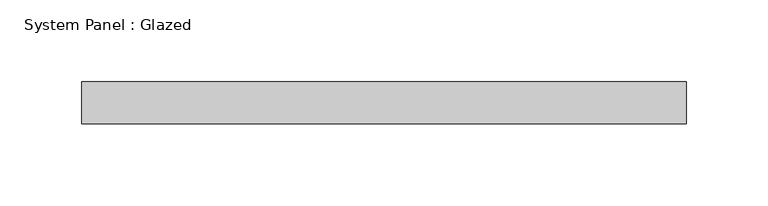
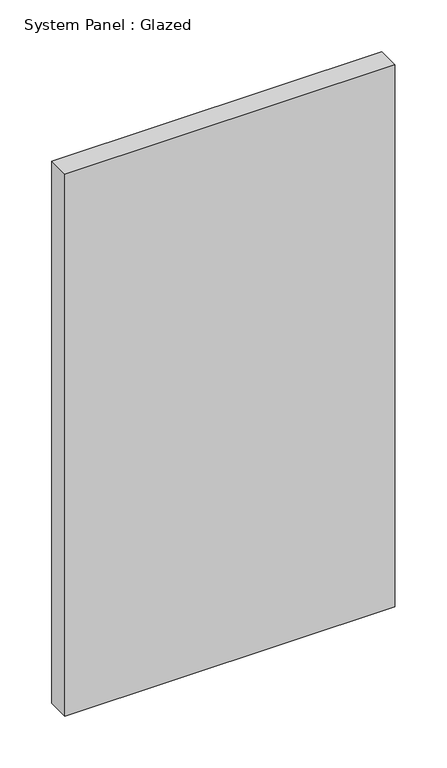
"""IFC4 building model written with IfcOpenShell, lengths in millimetres: plate geometry, System Panel : Glazed."""

from ifc_helpers import new_model, si_unit, origin, origin_with_axes, place, context, project, spatial, polyline, outline, extrude, source, transform, mapped, element, save


def system_panel_glazed_31ef28de(model_context):
    return source(origin(), model_context, "Body", "SweptSolid", [
        extrude(outline(polyline([(184.15, 19.05), (-184.15, 19.05), (-184.15, 44.45), (184.15, 44.45), (184.15, 19.05)])), origin_with_axes(), (0.0, 0.0, 1.0), 639.5466705),
    ])


if __name__ == "__main__":
    model = new_model("IFC4")
    model_context = context("Model", 3, world=origin())
    ifc_project = project(units=[si_unit("LENGTHUNIT", "METRE", prefix="MILLI")], contexts=[model_context])
    site = spatial("IfcSite", under=ifc_project)
    building = spatial("IfcBuilding", under=site)
    placement = place(None, origin())
    system_panel_glazed_shape = system_panel_glazed_31ef28de(model_context)
    element("IfcPlate", 1, ObjectType="System Panel : Glazed", at=placement, inside=building, context=model_context, shape_type="MappedRepresentation", body=[
        mapped(system_panel_glazed_shape, transform((0.0, 0.0, 0.0), x_axis=(1.0, 0.0, 0.0), y_axis=(0.0, 1.0, 0.0), z_axis=(0.0, 0.0, 1.0))),
    ])
    save(model, "model.ifc")

# Revit data of these elements
# Type "System Panel : Glazed"
#   Construction Type Id = "GSP4R"
#   Analytic Construction = "1/8 in Pilkington single glazing"
#   Visual Light Transmittance = 0.9
#   Solar Heat Gain Coefficient = 0.86
#   Heat Transfer Coefficient (U) = 1.18115 BTU/(h·ft²·°F)
#   Define Thermal Properties by = 1
# Element 1 (IfcPlate, "System Panel : Glazed")
#   Materials on its faces: "Glass"
# Materials
#   "Glass": class "Glass", colour RGB 0 128 192, transparency 0.75, Description = "Soda Lime Glass", Cost = 0
